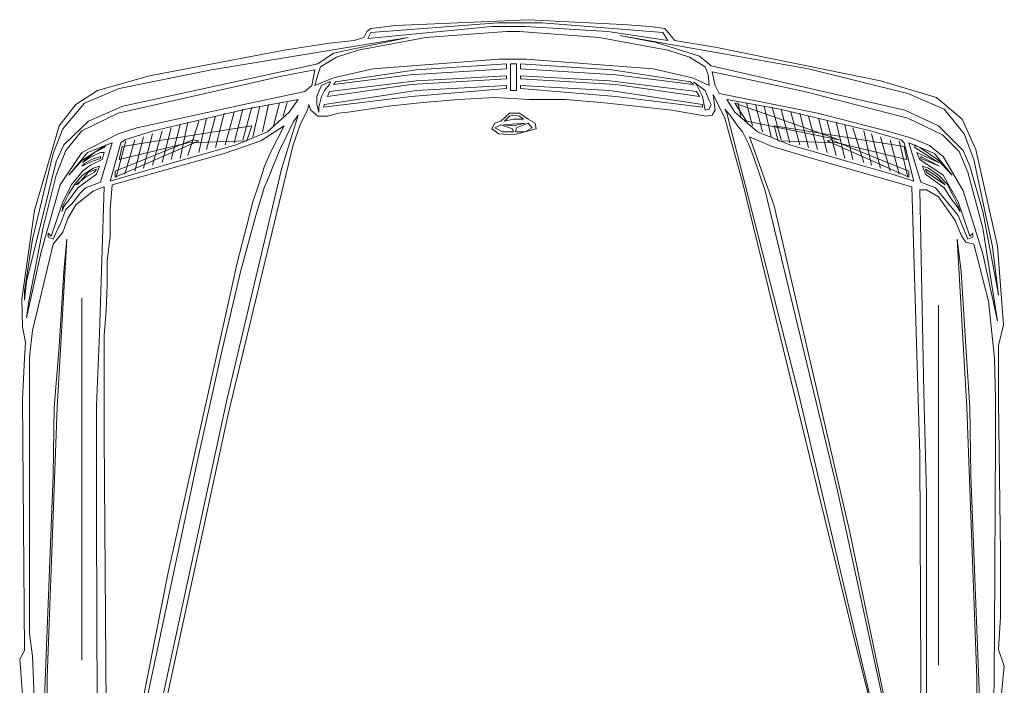
# Model space of a CAD drawing. Units: inches. Extents: x -36302355 to 648, y -221479757 to 75.
# Tile 10 of 37: x 185 to 224, y -455 to -428. Entities that reach past the tile are written whole.
import ezdxf

# ---------------------------------------------------------------- set-up
doc = ezdxf.new("R2010")
doc.units = ezdxf.units.IN
doc.header["$MEASUREMENT"] = 0
doc.layers.add('A-EQPM-VEHC', color=8, linetype='Continuous', lineweight=13)

msp = doc.modelspace()

# ---------------------------------------------------------------- linework, layer by layer
at = {"layer": 'A-EQPM-VEHC'}
for p, q in [((203.864, -428.585), (198.909, -429.057)), ((199.027, -428.822), (204.1, -428.429)), ((200.011, -428.546), (199.027, -428.664)), ((205.319, -428.31), (200.011, -428.546)), ((205.201, -428.585), (203.864, -428.585)), ((204.1, -428.429), (205.87, -428.429)), ((208.504, -428.782), (205.201, -428.585)), ((209.094, -428.508), (205.319, -428.31)), ((205.87, -428.429), (210.706, -428.822)), ((210.195, -428.585), (209.094, -428.508)), ((210.785, -428.664), (210.195, -428.585)), ((192.657, -430.315), (200.522, -429.018)), ((200.522, -429.018), (197.533, -429.647)), ((198.751, -429.018), (198.358, -429.136)), ((198.516, -429.529), (201.229, -429.018)), ((198.871, -428.782), (198.751, -429.018)), ((199.027, -428.664), (198.871, -428.782)), ((198.909, -429.057), (199.027, -428.822)), ((201.229, -429.018), (204.454, -428.782)), ((204.454, -428.782), (204.965, -428.782)), ((204.965, -428.782), (208.15, -429.018)), ((208.15, -429.018), (210.903, -429.529)), ((210.903, -429.136), (208.504, -428.782)), ((216.526, -430.277), (208.976, -428.94)), ((208.976, -428.94), (210.431, -429.215)), ((210.706, -428.822), (210.903, -429.136)), ((211.178, -429.136), (210.785, -428.664)), ((197.376, -429.254), (195.567, -429.529)), ((198.358, -429.136), (197.376, -429.254)), ((210.431, -429.215), (212.161, -429.766)), ((212.791, -429.412), (211.178, -429.136)), ((219.397, -430.749), (212.791, -429.412)), ((195.567, -429.529), (190.18, -430.552)), ((197.533, -429.647), (196.904, -430.08)), ((197.021, -430.198), (197.651, -429.805)), ((197.651, -429.805), (198.516, -429.529)), ((210.903, -429.529), (211.768, -429.805)), ((211.768, -429.805), (212.398, -430.198)), ((212.161, -429.766), (212.633, -430.159)), ((196.904, -430.08), (189.118, -431.772)), ((196.904, -430.512), (197.021, -430.198)), ((204.14, -429.884), (199.106, -430.277)), ((200.836, -430.315), (204.454, -430.08)), ((205.24, -429.884), (204.14, -429.884)), ((204.454, -430.08), (204.454, -430.277)), ((204.847, -430.08), (204.612, -430.08)), ((204.612, -430.08), (204.612, -431.142)), ((204.847, -431.142), (204.847, -430.08)), ((208.662, -430.315), (205.005, -430.08)), ((205.005, -430.08), (205.005, -430.277)), ((210.313, -430.277), (205.24, -429.884)), ((212.398, -430.198), (212.515, -430.512)), ((212.633, -430.159), (220.38, -431.928)), ((190.18, -430.552), (188.095, -431.142)), ((188.921, -432.045), (195.528, -430.552)), ((188.96, -431.063), (192.657, -430.315)), ((195.528, -430.552), (196.786, -430.315)), ((196.786, -430.315), (196.668, -430.945)), ((196.786, -430.945), (196.904, -430.512)), ((199.106, -430.277), (197.533, -430.631)), ((200.601, -430.512), (197.533, -430.906)), ((197.612, -430.787), (200.836, -430.315)), ((204.454, -430.277), (200.601, -430.512)), ((200.836, -430.749), (204.454, -430.552)), ((204.454, -430.552), (204.454, -430.67)), ((205.005, -430.277), (208.818, -430.512)), ((208.583, -430.749), (205.005, -430.552)), ((205.005, -430.552), (205.005, -430.67)), ((211.808, -430.787), (208.662, -430.315)), ((208.818, -430.512), (211.926, -430.906)), ((211.885, -430.631), (210.313, -430.277)), ((212.515, -430.512), (212.554, -430.945)), ((213.814, -430.631), (212.673, -430.394)), ((212.673, -430.394), (212.791, -430.945)), ((220.497, -431.259), (216.526, -430.277)), ((196.668, -430.945), (196.393, -431.18)), ((197.533, -430.631), (196.786, -430.945)), ((197.061, -430.945), (196.944, -431.18)), ((197.376, -430.787), (197.061, -430.945)), ((197.179, -431.142), (197.376, -430.906)), ((200.639, -430.906), (197.297, -431.377)), ((197.376, -431.18), (200.836, -430.749)), ((197.376, -430.906), (197.416, -430.787)), ((197.416, -430.787), (197.376, -430.787)), ((197.533, -430.906), (197.612, -430.787)), ((204.454, -430.67), (200.639, -430.906)), ((200.836, -431.142), (204.454, -430.945)), ((204.454, -430.945), (204.454, -431.063)), ((205.005, -430.67), (208.818, -430.906)), ((208.583, -431.142), (205.005, -430.945)), ((205.005, -430.945), (205.005, -431.063)), ((212.043, -431.18), (208.583, -430.749)), ((208.818, -430.906), (212.161, -431.377)), ((211.926, -430.906), (211.808, -430.787)), ((212.554, -430.945), (211.885, -430.631)), ((212.398, -431.142), (211.926, -430.787)), ((211.926, -430.787), (212.043, -430.906)), ((212.043, -430.906), (212.28, -431.377)), ((212.791, -430.945), (212.948, -431.259)), ((216.369, -431.18), (213.814, -430.631)), ((221.638, -431.417), (219.397, -430.749)), ((188.095, -431.142), (187.23, -431.693)), ((187.584, -431.652), (188.96, -431.063)), ((196.393, -431.18), (193.954, -431.693)), ((196.944, -431.18), (196.865, -431.377)), ((196.865, -431.377), (196.865, -431.693)), ((196.944, -431.81), (197.061, -431.377)), ((197.061, -431.377), (197.179, -431.142)), ((200.639, -431.377), (197.14, -431.81)), ((197.179, -431.693), (200.836, -431.142)), ((197.297, -431.377), (197.376, -431.18)), ((204.454, -431.063), (200.639, -431.377)), ((204.612, -431.142), (204.847, -431.142)), ((205.005, -431.063), (208.818, -431.377)), ((212.28, -431.693), (208.583, -431.142)), ((208.818, -431.377), (212.28, -431.81)), ((212.161, -431.377), (212.043, -431.18)), ((212.28, -431.377), (212.398, -431.928)), ((212.554, -431.535), (212.398, -431.142)), ((213.184, -432.242), (212.712, -431.3)), ((212.712, -431.3), (212.791, -431.928)), ((212.948, -431.259), (216.881, -432.045)), ((220.497, -432.242), (216.369, -431.18)), ((221.952, -431.889), (220.497, -431.259)), ((187.23, -431.693), (186.561, -432.558)), ((186.719, -432.675), (187.584, -431.652)), ((189.118, -431.772), (187.742, -432.361)), ((193.954, -431.693), (189.669, -432.637)), ((194.033, -431.889), (196.117, -431.496)), ((194.308, -432.989), (194.584, -431.772)), ((194.701, -432.793), (194.938, -431.693)), ((195.135, -432.558), (195.37, -431.652)), ((195.528, -432.165), (195.686, -431.614)), ((196.117, -431.496), (195.763, -432.007)), ((196.551, -431.693), (196.511, -431.889)), ((196.628, -431.928), (196.551, -431.693)), ((196.865, -431.693), (196.944, -432.007)), ((197.14, -431.81), (197.179, -431.693)), ((199.736, -431.772), (198.123, -432.007)), ((201.111, -431.614), (199.736, -431.772)), ((202.527, -431.496), (201.111, -431.614)), ((203.982, -431.417), (202.527, -431.496)), ((205.358, -431.496), (203.982, -431.417)), ((206.814, -431.496), (205.358, -431.496)), ((208.228, -431.614), (206.814, -431.496)), ((209.606, -431.772), (208.228, -431.614)), ((211.06, -431.928), (209.606, -431.772)), ((212.28, -431.81), (212.28, -431.693)), ((212.633, -431.693), (212.554, -431.535)), ((212.554, -431.889), (212.633, -431.693)), ((215.386, -431.889), (213.263, -431.496)), ((213.263, -431.496), (213.577, -432.007)), ((217.746, -433.107), (213.577, -431.652)), ((213.577, -431.652), (214.049, -432.361)), ((213.814, -432.165), (213.694, -431.614)), ((214.284, -432.558), (214.049, -431.652)), ((214.679, -432.793), (214.403, -431.693)), ((215.031, -432.989), (214.756, -431.772)), ((222.661, -432.282), (221.638, -431.417)), ((187.467, -432.754), (188.921, -432.045)), ((190.337, -432.754), (194.033, -431.889)), ((192.461, -433.502), (192.815, -432.165)), ((192.815, -433.423), (193.168, -432.045)), ((193.208, -433.305), (193.561, -432.007)), ((193.561, -433.226), (193.915, -431.889)), ((193.915, -433.107), (194.27, -431.81)), ((195.763, -432.007), (194.898, -432.793)), ((195.449, -434.288), (196.117, -432.124)), ((196.117, -432.124), (195.921, -432.4)), ((196.511, -431.889), (196.196, -432.517)), ((196.904, -432.165), (196.628, -431.928)), ((197.297, -432.165), (196.904, -432.165)), ((196.944, -432.007), (196.944, -431.81)), ((197.73, -432.045), (197.297, -432.165)), ((198.123, -432.007), (197.73, -432.045)), ((204.572, -432.045), (204.217, -432.361)), ((204.572, -432.165), (204.375, -432.361)), ((204.965, -432.045), (204.572, -432.045)), ((204.729, -432.124), (204.572, -432.165)), ((204.965, -432.165), (204.729, -432.124)), ((205.319, -432.282), (204.965, -432.045)), ((205.123, -432.282), (204.965, -432.165)), ((212.436, -432.165), (211.06, -431.928)), ((212.398, -431.928), (212.554, -431.889)), ((212.673, -432.124), (212.436, -432.165)), ((212.791, -431.928), (212.673, -432.124)), ((213.419, -432.165), (213.184, -431.889)), ((213.184, -431.889), (213.263, -432.045)), ((213.263, -432.045), (216.133, -443.293)), ((213.656, -432.517), (213.419, -432.165)), ((213.577, -432.007), (214.481, -432.793)), ((215.425, -433.107), (215.072, -431.81)), ((219.004, -432.754), (215.386, -431.889)), ((215.779, -433.226), (215.425, -431.889)), ((216.172, -433.305), (215.818, -432.007)), ((216.526, -433.423), (216.172, -432.045)), ((216.881, -433.502), (216.526, -432.165)), ((216.881, -432.045), (219.632, -432.754)), ((220.38, -431.928), (221.717, -432.558)), ((222.74, -432.872), (221.952, -431.889)), ((186.561, -432.558), (185.579, -435.939)), ((187.742, -432.361), (186.758, -433.305)), ((189.079, -433.383), (194.27, -432.558)), ((191.045, -433.895), (191.399, -432.517)), ((191.399, -433.855), (191.713, -432.4)), ((191.713, -433.737), (192.146, -432.361)), ((192.146, -433.619), (192.461, -432.242)), ((194.27, -432.558), (194.073, -433.147)), ((195.567, -432.558), (194.623, -433.147)), ((195.017, -433.619), (195.567, -432.558)), ((195.921, -432.4), (195.645, -432.989)), ((196.196, -432.517), (195.921, -433.305)), ((203.982, -432.44), (203.864, -432.675)), ((204.217, -432.361), (203.982, -432.44)), ((204.217, -432.517), (203.982, -432.637)), ((204.689, -432.675), (204.217, -432.517)), ((205.201, -432.44), (204.336, -432.517)), ((204.336, -432.517), (204.729, -432.558)), ((204.375, -432.361), (204.729, -432.282)), ((204.729, -432.282), (205.123, -432.282)), ((204.729, -432.558), (205.201, -432.44)), ((205.319, -432.44), (204.847, -432.637)), ((205.595, -432.44), (205.319, -432.282)), ((205.477, -432.637), (205.319, -432.44)), ((205.633, -432.675), (205.595, -432.44)), ((213.891, -434.799), (213.184, -432.242)), ((213.891, -432.793), (213.656, -432.517)), ((214.049, -432.361), (217.746, -433.107)), ((220.341, -433.383), (215.149, -432.558)), ((215.149, -432.558), (215.307, -433.147)), ((217.274, -433.619), (216.919, -432.242)), ((217.627, -433.737), (217.274, -432.361)), ((217.981, -433.855), (217.627, -432.4)), ((218.295, -433.895), (217.981, -432.517)), ((221.875, -432.911), (220.497, -432.242)), ((221.717, -432.558), (222.7, -433.54)), ((223.212, -433.502), (222.661, -432.282)), ((186.326, -433.658), (186.719, -432.675)), ((186.837, -433.54), (187.467, -432.754)), ((188.921, -432.872), (187.467, -433.619)), ((189.669, -432.637), (188.921, -432.872)), ((189.197, -433.107), (190.337, -432.754)), ((189.944, -434.248), (190.297, -432.872)), ((190.297, -434.13), (190.69, -432.754)), ((190.69, -434.012), (191.045, -432.637)), ((194.898, -432.793), (193.64, -433.305)), ((203.864, -432.675), (204.14, -432.872)), ((203.982, -432.637), (204.296, -432.793)), ((204.14, -432.872), (204.729, -432.911)), ((204.296, -432.793), (204.729, -432.793)), ((204.729, -432.793), (204.689, -432.675)), ((204.729, -432.911), (205.633, -432.675)), ((204.847, -432.637), (204.808, -432.793)), ((204.808, -432.793), (205.201, -432.793)), ((205.201, -432.793), (205.477, -432.637)), ((214.128, -433.265), (213.891, -432.793)), ((214.481, -432.793), (215.779, -433.305)), ((218.729, -434.012), (218.295, -432.637)), ((219.043, -434.13), (218.729, -432.754)), ((220.222, -433.107), (219.004, -432.754)), ((219.397, -434.248), (219.043, -432.872)), ((219.632, -432.754), (220.615, -433.03)), ((222.543, -433.579), (221.875, -432.911)), ((223.133, -433.895), (222.74, -432.872)), ((186.758, -433.305), (186.444, -433.972)), ((187.702, -433.619), (188.686, -433.226)), ((188.686, -433.226), (188.214, -434.799)), ((188.449, -433.305), (188.292, -433.423)), ((188.37, -433.423), (188.449, -433.305)), ((188.607, -434.76), (189.039, -433.226)), ((188.804, -434.367), (191.91, -433.107)), ((192.146, -433.147), (188.804, -434.602)), ((188.842, -434.602), (189.236, -433.147)), ((191.713, -433.226), (188.96, -433.895)), ((189.039, -433.226), (189.197, -433.107)), ((189.197, -434.484), (189.59, -433.107)), ((189.59, -434.367), (189.944, -432.989)), ((193.64, -433.305), (191.281, -433.972)), ((194.073, -433.147), (191.713, -433.226)), ((191.91, -433.107), (192.146, -433.147)), ((194.623, -433.147), (193.168, -433.658)), ((195.921, -433.305), (193.326, -444.079)), ((195.645, -432.989), (195.37, -433.54)), ((214.324, -433.776), (214.128, -433.265)), ((215.072, -433.383), (214.166, -432.989)), ((214.166, -432.989), (215.149, -435.743)), ((215.307, -433.147), (217.667, -433.226)), ((215.779, -433.305), (218.099, -433.972)), ((217.43, -433.107), (217.274, -433.147)), ((217.274, -433.147), (220.538, -434.602)), ((220.538, -434.367), (217.43, -433.107)), ((217.667, -433.226), (220.459, -433.895)), ((219.79, -434.367), (219.397, -432.989)), ((220.145, -434.484), (219.79, -433.107)), ((220.497, -434.602), (220.145, -433.147)), ((220.341, -433.226), (220.222, -433.107)), ((220.734, -434.76), (220.341, -433.226)), ((221.559, -433.658), (220.538, -433.226)), ((220.538, -433.226), (221.01, -434.799)), ((220.615, -433.03), (221.362, -433.344)), ((220.773, -433.423), (220.773, -433.305)), ((220.773, -433.305), (220.969, -433.423)), ((221.362, -433.344), (221.913, -433.776)), ((185.5, -437.08), (186.326, -433.658)), ((186.444, -434.523), (186.837, -433.54)), ((187.467, -433.619), (186.602, -434.916)), ((186.954, -434.523), (187.702, -433.619)), ((188.292, -433.423), (187.467, -433.933)), ((187.623, -433.895), (187.977, -433.619)), ((188.214, -433.619), (187.86, -433.776)), ((187.977, -433.619), (188.37, -433.423)), ((188.37, -433.619), (188.214, -433.619)), ((188.292, -433.895), (188.37, -433.619)), ((193.168, -433.658), (188.686, -434.916)), ((188.96, -433.895), (189.079, -433.383)), ((194.78, -434.17), (195.017, -433.619)), ((195.37, -433.54), (195.135, -434.13)), ((216.683, -433.855), (215.072, -433.383)), ((220.459, -433.895), (220.341, -433.383)), ((221.717, -434.012), (220.773, -433.423)), ((220.969, -433.895), (220.852, -433.619)), ((220.852, -433.619), (221.717, -434.012)), ((220.969, -433.423), (221.678, -433.895)), ((222.268, -434.523), (221.559, -433.658)), ((222.896, -434.405), (222.543, -433.579)), ((222.7, -433.54), (222.975, -434.17)), ((224.077, -437.355), (223.212, -433.502)), ((186.444, -433.972), (185.265, -438.771)), ((187.467, -433.933), (186.954, -434.523)), ((187.86, -433.972), (187.467, -434.17)), ((187.467, -434.17), (187.584, -434.051)), ((187.86, -433.776), (187.505, -434.012)), ((187.505, -434.012), (187.623, -433.895)), ((187.505, -434.367), (187.821, -434.13)), ((187.584, -434.051), (187.86, -433.895)), ((187.821, -434.13), (188.292, -433.895)), ((187.86, -433.895), (188.214, -433.776)), ((188.214, -433.855), (187.86, -433.972)), ((188.214, -433.776), (188.214, -433.855)), ((191.281, -433.972), (189.551, -434.484)), ((195.135, -434.13), (194.898, -434.72)), ((214.559, -434.484), (214.324, -433.776)), ((220.655, -434.995), (216.683, -433.855)), ((218.099, -433.972), (219.869, -434.484)), ((221.913, -434.523), (220.969, -433.895)), ((221.01, -433.776), (221.01, -433.855)), ((221.756, -434.17), (221.01, -433.776)), ((221.01, -433.855), (221.756, -434.17)), ((221.678, -433.895), (222.268, -434.523)), ((221.913, -433.776), (222.7, -435.153)), ((223.879, -437.394), (223.133, -433.895)), ((185.933, -436.608), (186.444, -434.523)), ((187.191, -434.877), (187.505, -434.523)), ((187.309, -434.602), (187.505, -434.367)), ((187.309, -434.877), (187.742, -434.405)), ((188.056, -434.484), (187.309, -435.035)), ((187.505, -434.523), (187.939, -434.248)), ((187.977, -434.405), (187.623, -434.602)), ((187.742, -434.405), (188.056, -434.288)), ((187.939, -434.248), (188.174, -434.17)), ((188.056, -434.288), (187.977, -434.405)), ((188.174, -434.17), (188.056, -434.484)), ((189.551, -434.484), (188.607, -434.76)), ((188.804, -434.602), (188.804, -434.367)), ((193.287, -443.449), (195.449, -434.288)), ((194.545, -434.877), (194.78, -434.17)), ((214.796, -435.153), (214.559, -434.484)), ((219.869, -434.484), (220.734, -434.76)), ((220.538, -434.602), (220.538, -434.367)), ((221.324, -434.248), (221.087, -434.17)), ((221.087, -434.17), (221.206, -434.484)), ((221.638, -434.563), (221.206, -434.288)), ((221.206, -434.288), (221.245, -434.405)), ((221.206, -434.484), (221.952, -435.035)), ((221.245, -434.405), (221.992, -434.916)), ((221.717, -434.523), (221.324, -434.248)), ((222.071, -434.877), (221.717, -434.523)), ((222.503, -435.585), (221.913, -434.523)), ((223.486, -436.646), (222.896, -434.405)), ((222.975, -434.17), (223.486, -435.978)), ((186.602, -434.916), (185.854, -437.59)), ((186.719, -435.585), (187.074, -434.877)), ((186.954, -435.271), (187.191, -434.877)), ((187.074, -434.877), (187.309, -434.602)), ((187.623, -434.602), (187.23, -434.916)), ((187.23, -434.916), (187.309, -434.877)), ((187.939, -434.916), (187.623, -435.035)), ((188.214, -434.799), (187.939, -434.916)), ((188.686, -434.916), (188.607, -435.9)), ((194.308, -435.585), (194.545, -434.877)), ((194.898, -434.72), (194.78, -434.995)), ((215.818, -442.703), (213.891, -434.799)), ((221.01, -434.799), (221.599, -435.035)), ((221.992, -434.916), (221.638, -434.563)), ((222.268, -435.271), (222.071, -434.877)), ((186.719, -435.743), (186.954, -435.271)), ((187.309, -435.035), (186.995, -435.467)), ((187.939, -435.153), (187.23, -435.704)), ((187.426, -435.232), (187.23, -435.467)), ((187.623, -435.035), (187.426, -435.232)), ((188.37, -434.995), (187.939, -435.153)), ((188.174, -440.854), (188.37, -434.995)), ((194.78, -434.995), (194.426, -436.136)), ((217.667, -447.067), (214.796, -435.153)), ((220.969, -445.692), (220.655, -434.995)), ((221.245, -435.113), (220.969, -435.113)), ((220.969, -435.113), (221.127, -443.214)), ((221.717, -435.388), (221.245, -435.113)), ((221.599, -435.035), (222.503, -436.136)), ((221.952, -435.035), (222.228, -435.467)), ((222.503, -435.743), (222.268, -435.271)), ((222.7, -435.153), (223.486, -437.669)), ((186.444, -436.372), (186.719, -435.585)), ((186.995, -435.467), (186.758, -435.781)), ((187.074, -435.664), (186.837, -435.9)), ((187.23, -435.704), (186.916, -436.253)), ((187.23, -435.467), (187.074, -435.664)), ((194.073, -436.529), (194.308, -435.585)), ((222.385, -436.332), (221.717, -435.388)), ((222.228, -435.467), (222.464, -435.781)), ((222.975, -436.962), (222.503, -435.585)), ((185.579, -435.939), (185.068, -439.478)), ((186.681, -435.978), (186.719, -435.743)), ((186.758, -435.781), (186.681, -435.978)), ((186.837, -435.9), (186.719, -436.215)), ((188.607, -435.9), (188.607, -436.962)), ((215.149, -435.743), (218.178, -448.798)), ((222.464, -435.781), (222.582, -435.978)), ((222.582, -435.978), (222.503, -435.743)), ((223.486, -435.978), (224.077, -439.085)), ((186.247, -436.962), (186.444, -436.372)), ((186.602, -436.49), (186.484, -436.725)), ((186.719, -436.215), (186.602, -436.49)), ((186.916, -436.253), (186.719, -436.804)), ((194.426, -436.136), (194.152, -437.159)), ((222.621, -436.922), (222.385, -436.332)), ((222.503, -436.136), (222.896, -437.08)), ((185.343, -439.636), (185.933, -436.608)), ((186.13, -437.001), (186.13, -436.843)), ((186.13, -436.843), (186.247, -436.962)), ((186.484, -436.725), (186.326, -437.08)), ((186.719, -436.804), (186.326, -437.276)), ((193.68, -438.024), (194.073, -436.529)), ((223.093, -436.843), (222.975, -436.962)), ((223.093, -437.001), (223.093, -436.843)), ((223.998, -439.833), (223.486, -436.646)), ((185.224, -438.889), (185.5, -437.08)), ((186.326, -437.276), (185.5, -440.736)), ((186.326, -437.08), (186.13, -437.001)), ((186.484, -443.804), (186.877, -437.08)), ((186.877, -437.08), (186.758, -438.376)), ((188.607, -436.962), (188.488, -437.945)), ((194.152, -437.159), (193.836, -438.338)), ((222.857, -443.804), (222.464, -437.08)), ((222.464, -437.08), (222.621, -438.376)), ((222.817, -437.197), (222.621, -436.922)), ((223.133, -437.276), (222.817, -437.197)), ((222.896, -437.08), (223.093, -437.001)), ((223.722, -439.557), (223.133, -437.276)), ((185.854, -437.59), (185.265, -440.226)), ((223.486, -437.669), (224.077, -440.343)), ((224.116, -439.32), (223.879, -437.394)), ((224.312, -440.501), (224.077, -437.355)), ((188.488, -437.945), (188.488, -438.889)), ((193.287, -439.833), (193.68, -438.024)), ((186.758, -438.376), (186.561, -441.366)), ((193.836, -438.338), (193.05, -441.68)), ((222.621, -438.376), (222.817, -441.366)), ((185.265, -438.771), (185.186, -439.517)), ((185.186, -439.164), (185.224, -438.889)), ((185.186, -439.517), (185.186, -439.164)), ((188.488, -438.889), (188.449, -439.95)), ((224.077, -439.085), (224.116, -439.32)), ((185.068, -439.478), (185.107, -440.579)), ((185.265, -440.226), (185.343, -439.636)), ((187.467, -453.909), (187.467, -439.438)), ((223.958, -441.837), (223.722, -439.557)), ((188.449, -439.95), (188.37, -440.933)), ((190.927, -450.41), (193.287, -439.833)), ((221.717, -454.106), (221.717, -439.714)), ((224.077, -440.343), (223.998, -439.833)), ((185.107, -440.579), (185.224, -441.208)), ((185.5, -440.736), (185.382, -441.798)), ((224.116, -441.326), (224.312, -440.501)), ((185.224, -441.208), (185.186, -441.837)), ((188.056, -443.725), (188.174, -440.854)), ((188.37, -440.933), (188.37, -444.944)), ((186.561, -441.366), (186.365, -443.804)), ((222.817, -441.366), (222.975, -443.804)), ((224.116, -443.568), (224.116, -441.326)), ((185.186, -441.837), (185.107, -443.49)), ((185.382, -441.798), (185.382, -452.847)), ((193.05, -441.68), (192.068, -446.045)), ((223.998, -443.449), (223.958, -441.837)), ((218.374, -453.163), (215.818, -442.703)), ((185.107, -443.49), (185.186, -453.516)), ((190.101, -458.196), (193.287, -443.449)), ((216.133, -443.293), (219.515, -457.606)), ((221.127, -443.214), (221.245, -447.264)), ((223.998, -445.062), (223.998, -443.449)), ((224.194, -449.624), (224.116, -443.568)), ((186.089, -454.618), (186.484, -443.804)), ((186.365, -443.804), (186.326, -446.517)), ((188.056, -448.287), (188.056, -443.725)), ((223.25, -454.618), (222.857, -443.804)), ((222.975, -443.804), (223.014, -446.517)), ((193.326, -444.079), (190.69, -456.23)), ((188.37, -444.944), (188.449, -456.23)), ((223.958, -452.847), (223.998, -445.062)), ((221.01, -454.539), (220.969, -445.692)), ((192.068, -446.045), (189.669, -457.331)), ((186.326, -446.517), (185.972, -455.758)), ((223.014, -446.517), (223.368, -455.758)), ((220.341, -459.375), (217.667, -447.067)), ((221.245, -447.264), (221.245, -460.477)), ((188.095, -457.369), (188.056, -448.287)), ((218.178, -448.798), (220.341, -459.178)), ((224.194, -452.179), (224.194, -449.624)), ((189.551, -457.331), (190.927, -450.41)), ((224.116, -453.477), (224.194, -452.179)), ((185.382, -452.847), (185.5, -453.753)), ((223.879, -460.437), (223.958, -452.847)), ((219.515, -457.606), (218.374, -453.163)), ((185.186, -453.516), (184.989, -453.87)), ((185.5, -453.753), (185.579, -455.718)), ((224.351, -454.146), (224.116, -453.477)), ((184.989, -453.87), (185.186, -456.269)), ((224.233, -455.246), (224.351, -454.146)), ((186.089, -460.437), (186.089, -454.618)), ((220.969, -460.122), (221.01, -454.539)), ((223.25, -460.437), (223.25, -454.618))]:
    msp.add_line(p, q, dxfattribs=at)

doc.saveas('drawing.dxf')
